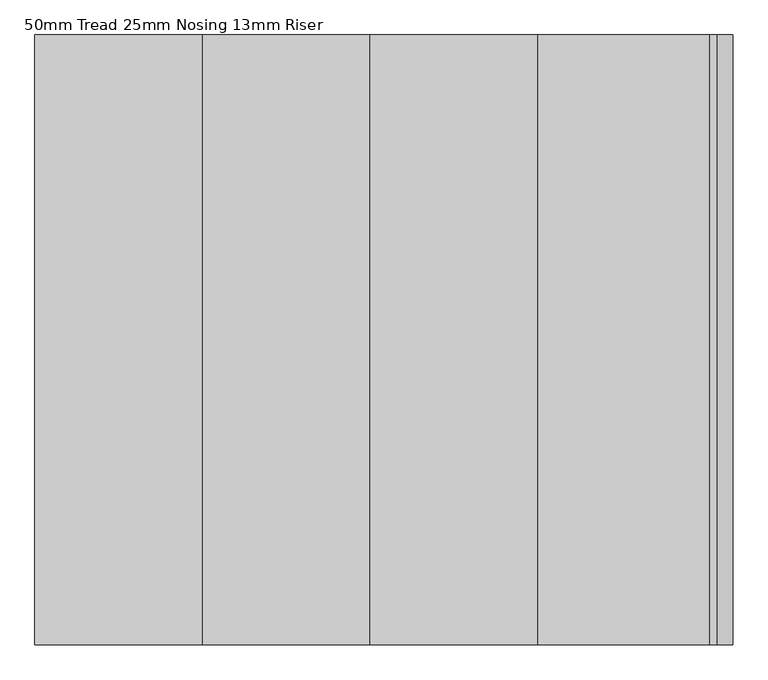
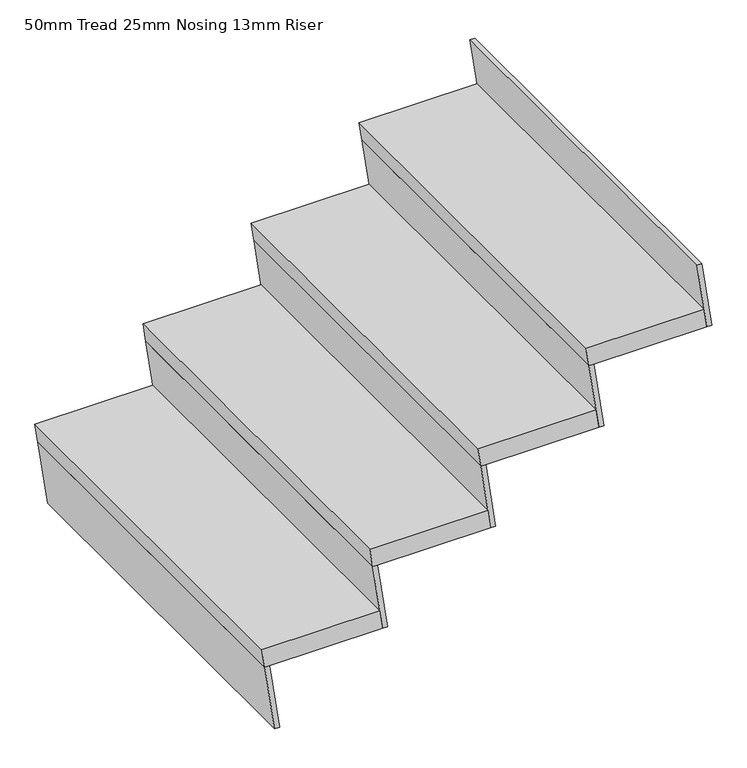
"""IFC4 building model written with IfcOpenShell, lengths in millimetres: stair flight geometry, 50mm Tread 25mm Nosing 13mm Riser."""

from ifc_helpers import new_model, si_unit, frame, origin, place, context, project, spatial, polyline, outline, extrude, source, transform, mapped, element, save


def stair_flight_50mm_tread_25mm_nosing_13mm_riser_f72ebc14(model_context):
    return source(origin(), model_context, "Body", "SweptSolid", [
        extrude(outline(polyline([(1217.3913043, -11114.1151057), (1217.3913043, -11414.1151057), (1167.3913043, -11406.9276057), (1167.3913043, -11106.9276057), (1217.3913043, -11114.1151057)])), frame((0.0, 2800.1398477, 0.0), z_axis=(0.0, 1.0, 0.0), x_axis=(0.0, 0.0, 1.0)), (0.0, 0.0, 1.0), 1000.0257813),
        extrude(outline(polyline([(1167.3913043, -11406.9276057), (993.4782609, -11381.9276057), (993.4782609, -11369.2991157), (1167.3913043, -11394.2991157), (1167.3913043, -11406.9276057)])), frame((0.0, 2800.1398477, 0.0), z_axis=(0.0, 1.0, 0.0), x_axis=(0.0, 0.0, 1.0)), (0.0, 0.0, 1.0), 1000.0257813),
        extrude(outline(polyline([(1341.3043478, -11131.9276057), (1167.3913043, -11106.9276057), (1167.3913043, -11094.2991157), (1341.3043478, -11119.2991157), (1341.3043478, -11131.9276057)])), frame((0.0, 2800.1398477, 0.0), z_axis=(0.0, 1.0, 0.0), x_axis=(0.0, 0.0, 1.0)), (0.0, 0.0, 1.0), 1000.0257813),
        extrude(outline(polyline([(1391.3043478, -10839.1151057), (1391.3043478, -11139.1151057), (1341.3043478, -11131.9276057), (1341.3043478, -10831.9276057), (1391.3043478, -10839.1151057)])), frame((0.0, 2800.1398477, 0.0), z_axis=(0.0, 1.0, 0.0), x_axis=(0.0, 0.0, 1.0)), (0.0, 0.0, 1.0), 1000.0257813),
        extrude(outline(polyline([(1515.2173913, -10856.9276057), (1341.3043478, -10831.9276057), (1341.3043478, -10819.2991157), (1515.2173913, -10844.2991157), (1515.2173913, -10856.9276057)])), frame((0.0, 2800.1398477, 0.0), z_axis=(0.0, 1.0, 0.0), x_axis=(0.0, 0.0, 1.0)), (0.0, 0.0, 1.0), 1000.0257813),
        extrude(outline(polyline([(1565.2173913, -10564.1151057), (1565.2173913, -10864.1151057), (1515.2173913, -10856.9276057), (1515.2173913, -10556.9276057), (1565.2173913, -10564.1151057)])), frame((0.0, 2800.1398477, 0.0), z_axis=(0.0, 1.0, 0.0), x_axis=(0.0, 0.0, 1.0)), (0.0, 0.0, 1.0), 1000.0257813),
        extrude(outline(polyline([(1689.1304348, -10581.9276057), (1515.2173913, -10556.9276057), (1515.2173913, -10544.2991157), (1689.1304348, -10569.2991157), (1689.1304348, -10581.9276057)])), frame((0.0, 2800.1398477, 0.0), z_axis=(0.0, 1.0, 0.0), x_axis=(0.0, 0.0, 1.0)), (0.0, 0.0, 1.0), 1000.0257813),
        extrude(outline(polyline([(1863.0434783, -10306.9276057), (1689.1304348, -10281.9276057), (1689.1304348, -10269.2991157), (1863.0434783, -10294.2991157), (1863.0434783, -10306.9276057)])), frame((0.0, 2800.1398477, 0.0), z_axis=(0.0, 1.0, 0.0), x_axis=(0.0, 0.0, 1.0)), (0.0, 0.0, 1.0), 1000.0257813),
        extrude(outline(polyline([(1739.1304348, -10289.1151057), (1739.1304348, -10589.1151057), (1689.1304348, -10581.9276057), (1689.1304348, -10281.9276057), (1739.1304348, -10289.1151057)])), frame((0.0, 2800.1398477, 0.0), z_axis=(0.0, 1.0, 0.0), x_axis=(0.0, 0.0, 1.0)), (0.0, 0.0, 1.0), 1000.0257813),
    ])


if __name__ == "__main__":
    model = new_model("IFC4")
    model_context = context("Model", 3, world=origin())
    ifc_project = project(units=[si_unit("LENGTHUNIT", "METRE", prefix="MILLI")], contexts=[model_context])
    site = spatial("IfcSite", under=ifc_project)
    building = spatial("IfcBuilding", under=site)
    placement = place(None, origin())
    stair_flight_50mm_tread_25mm_nosing_13mm_riser_shape = stair_flight_50mm_tread_25mm_nosing_13mm_riser_f72ebc14(model_context)
    element("IfcStairFlight", 1, ObjectType="50mm Tread 25mm Nosing 13mm Riser", at=placement, inside=building, context=model_context, shape_type="MappedRepresentation", body=[
        mapped(stair_flight_50mm_tread_25mm_nosing_13mm_riser_shape, transform((0.0, 0.0, 0.0), x_axis=(1.0, 0.0, 0.0), y_axis=(0.0, 1.0, 0.0), z_axis=(0.0, 0.0, 1.0))),
    ])
    save(model, "model.ifc")
